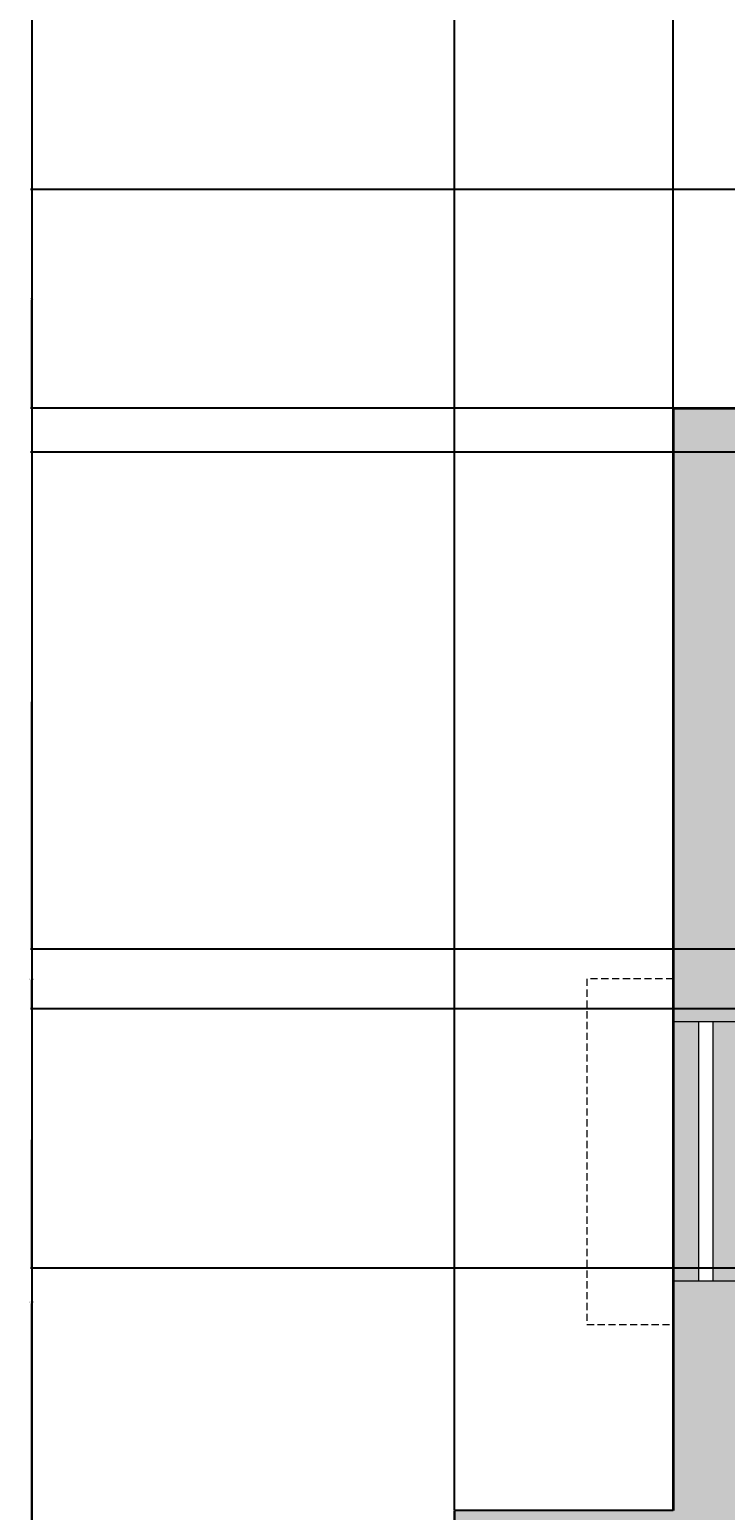
# Model space of a CAD drawing. Units: inches. Extents: x 1693 to 2974, y 2201 to 2965.
# Tile 4 of 24: x 1693 to 1790, y 2554 to 2759. Entities that reach past the tile are written whole.
import ezdxf

# ---------------------------------------------------------------- set-up
doc = ezdxf.new("R2010")
doc.units = ezdxf.units.IN
doc.header["$LTSCALE"] = 2
doc.header["$MEASUREMENT"] = 0
doc.linetypes.add('HIDDEN', pattern=[0.375, 0.25, -0.125])
for name, color, linetype, lineweight in [('A-ANNO-DIMS', 2, 'Continuous', 18), ('A-FLOR-SHFT', 7, 'Continuous', 25), ('A-GLAZ', 4, 'Continuous', 18), ('A-GLAZ-OVHD', 8, 'HIDDEN', 13), ('A-WALL', 7, 'Continuous', 35)]:
    doc.layers.add(name, color=color, linetype=linetype, lineweight=lineweight)
doc.layers.add('A-GLAZ-PATT', color=141, linetype='Continuous', lineweight=13, true_color=0xadddf7)
doc.layers.add('A-WALL-PATT', color=251, linetype='Continuous', lineweight=13, true_color=0x636466)
doc.styles.get("Standard").update_dxf_attribs({"font": 'arial.ttf'})
doc.dimstyles.get("Standard").update_dxf_attribs({"dimtxt": 0.18, "dimasz": 0.18, "dimexe": 0.18, "dimexo": 0.0625, "dimgap": 0.09, "dimtad": 0, "dimtih": 1, "dimtoh": 1, "dimdec": 1, "dimzin": 0, "dimdsep": 46, "dimlunit": 3, "dimtxsty": 'Standard', "dimcen": 0.09, "dimadec": 0, "dimazin": 0, "dimtfac": 1, "dimtdec": 1, "dimtofl": 0, "dimtmove": 0, "dimatfit": 3, "dimfxl": 1, "dimtolj": 1, "dimtzin": 0, "dimarcsym": 0})

# ---------------------------------------------------------------- blocks, each defined once
blk = doc.blocks.new('WINDOW-HOOD-48IN')
at = {"ltscale": 2}
for p, q in [((12, 48), (0, 48)), ((0, 48), (0, 6)), ((12, 42), (12, 48)), ((0, 6), (0, 0)), ((0, 0), (12, 0))]:
    blk.add_line(p, q, dxfattribs=at)
blk = doc.blocks.new('*D81')
at = {"layer": 'A-ANNO-DIMS', "color": 0, "lineweight": -2, "ltscale": 2, "transparency": 16777216}
for p, q in [((1752.34, 2553.91), (1752.34, 2964.96)), ((1752.52, 2964.78), (2332.94, 2964.78)), ((2914.06, 2964.78), (2333.64, 2964.78)), ((2914.24, 2754.97), (2914.24, 2964.96))]:
    blk.add_line(p, q, dxfattribs=at)
at = {"layer": 'A-ANNO-DIMS', "color": 0, "ltscale": 2, "transparency": 16777216}
for points in [[(1752.52, 2964.81), (1752.52, 2964.75), (1752.34, 2964.78)], [(2914.06, 2964.81), (2914.06, 2964.75), (2914.24, 2964.78)]]:
    blk.add_solid(points, dxfattribs=at)
at = {"layer": 'Defpoints', "color": 0, "ltscale": 2, "transparency": 16777216}
for p in [(2914.24, 2964.78), (2914.24, 2754.9), (1752.34, 2553.84)]:
    blk.add_point(p, dxfattribs=at)
at = {"layer": 'A-ANNO-DIMS', "color": 0, "ltscale": 2, "transparency": 16777216, "insert": (2333.29, 2964.78), "char_height": 0.18, "attachment_point": 5}
blk.add_mtext('\\A1;1162', dxfattribs=at)
blk = doc.blocks.new('*D82')
at = {"layer": 'A-ANNO-DIMS', "color": 0, "lineweight": -2, "ltscale": 2, "transparency": 16777216}
for p, q in [((2615.67, 2906.08), (1693.46, 2906.08)), ((1693.64, 2905.9), (1693.64, 2582.94)), ((1693.64, 2259.62), (1693.64, 2582.58)), ((2096.17, 2259.44), (1693.46, 2259.44))]:
    blk.add_line(p, q, dxfattribs=at)
at = {"layer": 'A-ANNO-DIMS', "color": 0, "ltscale": 2, "transparency": 16777216}
for points in [[(1693.61, 2905.9), (1693.67, 2905.9), (1693.64, 2906.08)], [(1693.61, 2259.62), (1693.67, 2259.62), (1693.64, 2259.44)]]:
    blk.add_solid(points, dxfattribs=at)
at = {"layer": 'Defpoints', "color": 0, "ltscale": 2, "transparency": 16777216}
for p in [(1693.64, 2906.08), (2615.74, 2906.08), (2096.24, 2259.44)]:
    blk.add_point(p, dxfattribs=at)
at = {"layer": 'A-ANNO-DIMS', "color": 0, "ltscale": 2, "transparency": 16777216, "insert": (1693.64, 2582.76), "char_height": 0.18, "attachment_point": 5}
blk.add_mtext('\\A1;646.6', dxfattribs=at)
blk = doc.blocks.new('*D86')
at = {"layer": 'A-ANNO-DIMS', "color": 0, "lineweight": -2, "ltscale": 2, "transparency": 16777216}
for p, q in [((1782.67, 2706.84), (1693.46, 2706.84)), ((1693.64, 2706.66), (1693.64, 2498.53)), ((1693.64, 2290.02), (1693.64, 2498.16)), ((1782.67, 2289.84), (1693.46, 2289.84))]:
    blk.add_line(p, q, dxfattribs=at)
at = {"layer": 'A-ANNO-DIMS', "color": 0, "ltscale": 2, "transparency": 16777216}
for points in [[(1693.61, 2706.66), (1693.67, 2706.66), (1693.64, 2706.84)], [(1693.61, 2290.02), (1693.67, 2290.02), (1693.64, 2289.84)]]:
    blk.add_solid(points, dxfattribs=at)
at = {"layer": 'Defpoints', "color": 0, "ltscale": 2, "transparency": 16777216}
for p in [(1693.64, 2706.84), (1782.74, 2706.84), (1782.74, 2289.84)]:
    blk.add_point(p, dxfattribs=at)
at = {"layer": 'A-ANNO-DIMS', "color": 0, "ltscale": 2, "transparency": 16777216, "insert": (1693.64, 2498.34), "char_height": 0.18, "attachment_point": 5}
blk.add_mtext('\\A1;417', dxfattribs=at)
blk = doc.blocks.new('*D88')
at = {"layer": 'A-ANNO-DIMS', "color": 0, "lineweight": -2, "ltscale": 2, "transparency": 16777216}
for p, q in [((2479.17, 2700.75), (1693.46, 2700.75)), ((1693.64, 2700.57), (1693.64, 2666.44)), ((1693.64, 2631.93), (1693.64, 2666.07)), ((2479.17, 2631.75), (1693.46, 2631.75))]:
    blk.add_line(p, q, dxfattribs=at)
at = {"layer": 'A-ANNO-DIMS', "color": 0, "ltscale": 2, "transparency": 16777216}
for points in [[(1693.61, 2700.57), (1693.67, 2700.57), (1693.64, 2700.75)], [(1693.61, 2631.93), (1693.67, 2631.93), (1693.64, 2631.75)]]:
    blk.add_solid(points, dxfattribs=at)
at = {"layer": 'Defpoints', "color": 0, "ltscale": 2, "transparency": 16777216}
for p in [(1693.64, 2700.75), (2479.24, 2700.75), (2479.24, 2631.75)]:
    blk.add_point(p, dxfattribs=at)
at = {"layer": 'A-ANNO-DIMS', "color": 0, "ltscale": 2, "transparency": 16777216, "insert": (1693.64, 2666.25), "char_height": 0.18, "attachment_point": 5}
blk.add_mtext('\\A1;69', dxfattribs=at)
blk = doc.blocks.new('*D98')
at = {"layer": 'A-ANNO-DIMS', "color": 0, "lineweight": -2, "ltscale": 2, "transparency": 16777216}
for p, q in [((2479.17, 2623.46), (1693.46, 2623.46)), ((1693.64, 2623.28), (1693.64, 2605.64)), ((1693.64, 2587.64), (1693.64, 2605.28)), ((2479.17, 2587.46), (1693.46, 2587.46))]:
    blk.add_line(p, q, dxfattribs=at)
at = {"layer": 'A-ANNO-DIMS', "color": 0, "ltscale": 2, "transparency": 16777216}
for points in [[(1693.61, 2623.28), (1693.67, 2623.28), (1693.64, 2623.46)], [(1693.61, 2587.64), (1693.67, 2587.64), (1693.64, 2587.46)]]:
    blk.add_solid(points, dxfattribs=at)
at = {"layer": 'Defpoints', "color": 0, "ltscale": 2, "transparency": 16777216}
for p in [(1693.64, 2623.46), (2479.24, 2623.46), (2479.24, 2587.46)]:
    blk.add_point(p, dxfattribs=at)
at = {"layer": 'A-ANNO-DIMS', "color": 0, "ltscale": 2, "transparency": 16777216, "insert": (1693.64, 2605.46), "char_height": 0.18, "attachment_point": 5}
blk.add_mtext('\\A1;36', dxfattribs=at)
blk = doc.blocks.new('*D99')
at = {"layer": 'A-ANNO-DIMS', "color": 0, "lineweight": -2, "ltscale": 2, "transparency": 16777216}
for p, q in [((2479.17, 2631.75), (1693.46, 2631.75)), ((1693.64, 2631.57), (1693.64, 2627.79)), ((1693.64, 2623.64), (1693.64, 2627.43)), ((2479.17, 2623.46), (1693.46, 2623.46))]:
    blk.add_line(p, q, dxfattribs=at)
at = {"layer": 'A-ANNO-DIMS', "color": 0, "ltscale": 2, "transparency": 16777216}
for points in [[(1693.61, 2631.57), (1693.67, 2631.57), (1693.64, 2631.75)], [(1693.61, 2623.64), (1693.67, 2623.64), (1693.64, 2623.46)]]:
    blk.add_solid(points, dxfattribs=at)
at = {"layer": 'Defpoints', "color": 0, "ltscale": 2, "transparency": 16777216}
for p in [(1693.64, 2631.75), (2479.24, 2631.75), (2479.24, 2623.46)]:
    blk.add_point(p, dxfattribs=at)
at = {"layer": 'A-ANNO-DIMS', "color": 0, "ltscale": 2, "transparency": 16777216, "insert": (1693.64, 2627.61), "char_height": 0.18, "attachment_point": 5}
blk.add_mtext('\\A1;8.295', dxfattribs=at)
blk = doc.blocks.new('*D102')
at = {"layer": 'A-ANNO-DIMS', "color": 0, "lineweight": -2, "ltscale": 2, "transparency": 16777216}
for p, q in [((1782.74, 2706.91), (1782.74, 2964.96)), ((1782.92, 2964.78), (1852.97, 2964.78)), ((1923.56, 2964.78), (1853.5, 2964.78)), ((1923.74, 2706.91), (1923.74, 2964.96))]:
    blk.add_line(p, q, dxfattribs=at)
at = {"layer": 'A-ANNO-DIMS', "color": 0, "ltscale": 2, "transparency": 16777216}
for points in [[(1782.92, 2964.81), (1782.92, 2964.75), (1782.74, 2964.78)], [(1923.56, 2964.81), (1923.56, 2964.75), (1923.74, 2964.78)]]:
    blk.add_solid(points, dxfattribs=at)
at = {"layer": 'Defpoints', "color": 0, "ltscale": 2, "transparency": 16777216}
for p in [(1923.74, 2964.78), (1782.74, 2706.84), (1923.74, 2706.84)]:
    blk.add_point(p, dxfattribs=at)
at = {"layer": 'A-ANNO-DIMS', "color": 0, "ltscale": 2, "transparency": 16777216, "insert": (1853.24, 2964.78), "char_height": 0.18, "attachment_point": 5}
blk.add_mtext('\\A1;141', dxfattribs=at)
blk = doc.blocks.new('*D105')
at = {"layer": 'A-ANNO-DIMS', "color": 0, "lineweight": -2, "ltscale": 2, "transparency": 16777216}
for p, q in [((1923.67, 2737.22), (1693.46, 2737.22)), ((1693.64, 2737.04), (1693.64, 2722.21)), ((1693.64, 2707.02), (1693.64, 2721.85)), ((1923.67, 2706.84), (1693.46, 2706.84))]:
    blk.add_line(p, q, dxfattribs=at)
at = {"layer": 'A-ANNO-DIMS', "color": 0, "ltscale": 2, "transparency": 16777216}
for points in [[(1693.61, 2737.04), (1693.67, 2737.04), (1693.64, 2737.22)], [(1693.61, 2707.02), (1693.67, 2707.02), (1693.64, 2706.84)]]:
    blk.add_solid(points, dxfattribs=at)
at = {"layer": 'Defpoints', "color": 0, "ltscale": 2, "transparency": 16777216}
for p in [(1693.64, 2737.22), (1923.74, 2737.22), (1923.74, 2706.84)]:
    blk.add_point(p, dxfattribs=at)
at = {"layer": 'A-ANNO-DIMS', "color": 0, "ltscale": 2, "transparency": 16777216, "insert": (1693.64, 2722.03), "char_height": 0.18, "attachment_point": 5}
blk.add_mtext('\\A1;30.37', dxfattribs=at)

msp = doc.modelspace()

# ---------------------------------------------------------------- hatches: boundary and pattern name
at = {"layer": 'A-GLAZ-PATT', "ltscale": 2}
h = msp.add_hatch(color=256, dxfattribs=at)
h.dxf.hatch_style = 1
h.paths.add_polyline_path([(2656.9702, 2338.2547), (2632.9702, 2338.2547), (2632.9702, 2339.2547), (2608.9702, 2339.2547), (2608.9702, 2334.7547), (2656.9702, 2334.7547)])
h.paths.add_polyline_path([(2656.9702, 2343.7547), (2608.9702, 2343.7547), (2608.9702, 2340.2547), (2632.9702, 2340.2547), (2632.9702, 2339.2547), (2656.9702, 2339.2547)])
h.paths.add_polyline_path([(2775.7544, 2338.2547), (2751.7544, 2338.2547), (2751.7544, 2334.7547), (2775.7544, 2334.7547)])
h.paths.add_polyline_path([(2775.7544, 2343.7547), (2751.7544, 2343.7547), (2751.7544, 2340.2547), (2775.7544, 2340.2547)])
h.paths.add_polyline_path([(2897.7363, 2568.7999), (2893.2363, 2568.7999), (2893.2363, 2520.7999), (2896.7363, 2520.7999), (2896.7363, 2544.7999), (2897.7363, 2544.7999)])
h.paths.add_polyline_path([(2902.2363, 2568.7999), (2898.7363, 2568.7999), (2898.7363, 2544.7999), (2897.7363, 2544.7999), (2897.7363, 2520.7999), (2902.2363, 2520.7999)])
h.paths.add_polyline_path([(2902.2363, 2637.7547), (2898.7363, 2637.7547), (2898.7363, 2613.7547), (2902.2363, 2613.7547)])
h.paths.add_polyline_path([(2896.7363, 2637.7547), (2893.2363, 2637.7547), (2893.2363, 2613.7547), (2896.7363, 2613.7547)])
h.paths.add_polyline_path([(2902.2363, 2748.903), (2899.0477, 2748.903), (2899.0477, 2724.903), (2898.0477, 2724.903), (2898.0477, 2700.903), (2902.2363, 2700.903)])
h.paths.add_polyline_path([(2898.0477, 2748.903), (2893.2363, 2748.903), (2893.2363, 2700.903), (2897.0477, 2700.903), (2897.0477, 2724.903), (2898.0477, 2724.903)])
h.paths.add_polyline_path([(2851.2363, 2846.2547), (2803.2363, 2846.2547), (2803.2363, 2842.7547), (2827.2363, 2842.7547), (2827.2363, 2841.7547), (2851.2363, 2841.7547)])
h.paths.add_polyline_path([(2851.2363, 2840.7547), (2827.2363, 2840.7547), (2827.2363, 2841.7547), (2803.2363, 2841.7547), (2803.2363, 2837.2547), (2851.2363, 2837.2547)])
h.paths.add_polyline_path([(2578.2363, 2846.2547), (2530.2363, 2846.2547), (2530.2363, 2842.7547), (2554.2363, 2842.7547), (2554.2363, 2841.7547), (2578.2363, 2841.7547)])
h.paths.add_polyline_path([(2578.2363, 2840.7547), (2554.2363, 2840.7547), (2554.2363, 2841.7547), (2530.2363, 2841.7547), (2530.2363, 2837.2547), (2578.2363, 2837.2547)])
h.paths.add_polyline_path([(2732.7363, 2812.7547), (2705.1363, 2812.7547), (2705.1363, 2811.7547), (2676.3363, 2811.7547), (2676.3363, 2812.7547), (2648.7363, 2812.7547), (2648.7363, 2808.2547), (2732.7363, 2808.2547)])
h.paths.add_polyline_path([(2732.7363, 2817.2547), (2648.7363, 2817.2547), (2648.7363, 2813.7547), (2676.3363, 2813.7547), (2676.3363, 2812.7547), (2705.1363, 2812.7547), (2705.1363, 2813.7547), (2732.7363, 2813.7547)])
h.paths.add_polyline_path([(2488.2363, 2695.8203), (2484.7878, 2695.8203), (2484.7878, 2671.8203), (2488.2363, 2671.8203)])
h.paths.add_polyline_path([(2482.7878, 2695.8203), (2479.2363, 2695.8203), (2479.2363, 2671.8203), (2482.7878, 2671.8203)])
h.paths.add_polyline_path([(2488.2363, 2572.4371), (2484.7363, 2572.4371), (2484.7363, 2541.4371), (2483.7363, 2541.4371), (2483.7363, 2512.4371), (2488.2363, 2512.4371)])
h.paths.add_polyline_path([(2482.7363, 2541.4371), (2483.7363, 2541.4371), (2483.7363, 2572.4371), (2479.2363, 2572.4371), (2479.2363, 2512.4371), (2482.7363, 2512.4371)])
h.paths.add_polyline_path([(2248.9863, 2706.8449), (2190.9863, 2706.8449), (2190.9863, 2703.3449), (2219.9863, 2703.3449), (2219.9863, 2702.3449), (2248.9863, 2702.3449)])
h.paths.add_polyline_path([(2248.9863, 2701.3449), (2219.9863, 2701.3449), (2219.9863, 2702.3449), (2190.9863, 2702.3449), (2190.9863, 2697.8449), (2248.9863, 2697.8449)])
h.paths.add_polyline_path([(2151.9207, 2293.3449), (2127.9207, 2293.3449), (2127.9207, 2289.8449), (2151.9207, 2289.8449)])
h.paths.add_polyline_path([(2151.9207, 2298.8449), (2127.9207, 2298.8449), (2127.9207, 2295.3449), (2151.9207, 2295.3449)])
h.paths.add_polyline_path([(2084.023, 2293.3449), (2066.023, 2293.3449), (2066.023, 2294.3449), (2048.023, 2294.3449), (2048.023, 2289.8449), (2084.023, 2289.8449)])
h.paths.add_polyline_path([(2084.023, 2298.8449), (2048.023, 2298.8449), (2048.023, 2295.3449), (2066.023, 2295.3449), (2066.023, 2294.3449), (2084.023, 2294.3449)])
h.paths.add_polyline_path([(1966.0781, 2293.3449), (1948.0781, 2293.3449), (1948.0781, 2294.3449), (1930.0781, 2294.3449), (1930.0781, 2289.8449), (1966.0781, 2289.8449)])
h.paths.add_polyline_path([(1966.0781, 2298.8449), (1930.0781, 2298.8449), (1930.0781, 2295.3449), (1948.0781, 2295.3449), (1948.0781, 2294.3449), (1966.0781, 2294.3449)])
h.paths.add_polyline_path([(1787.2363, 2403.1922), (1782.7363, 2403.1922), (1782.7363, 2355.1922), (1786.2363, 2355.1922), (1786.2363, 2379.1922), (1787.2363, 2379.1922)])
h.paths.add_polyline_path([(1791.7363, 2403.1922), (1788.2363, 2403.1922), (1788.2363, 2379.1922), (1787.2363, 2379.1922), (1787.2363, 2355.1922), (1791.7363, 2355.1922)])
h.paths.add_polyline_path([(1786.2363, 2477.5455), (1782.7363, 2477.5455), (1782.7363, 2453.5455), (1786.2363, 2453.5455)])
h.paths.add_polyline_path([(1791.7363, 2477.5455), (1788.2363, 2477.5455), (1788.2363, 2453.5455), (1791.7363, 2453.5455)])
h.paths.add_polyline_path([(1786.2363, 2621.6433), (1782.7363, 2621.6433), (1782.7363, 2585.6433), (1786.2363, 2585.6433)])
h.paths.add_polyline_path([(1791.7363, 2621.6433), (1788.2363, 2621.6433), (1788.2363, 2585.6433), (1791.7363, 2585.6433)])
h.paths.add_polyline_path([(1908.1286, 2706.8449), (1860.1286, 2706.8449), (1860.1286, 2703.3449), (1884.1286, 2703.3449), (1884.1286, 2702.3449), (1908.1286, 2702.3449)])
h.paths.add_polyline_path([(1908.1286, 2701.3449), (1884.1286, 2701.3449), (1884.1286, 2702.3449), (1860.1286, 2702.3449), (1860.1286, 2697.8449), (1908.1286, 2697.8449)])
h.paths.add_polyline_path([(1973.9863, 2706.8449), (1949.9863, 2706.8449), (1949.9863, 2703.3449), (1973.9863, 2703.3449)])
h.paths.add_polyline_path([(1973.9863, 2701.3449), (1949.9863, 2701.3449), (1949.9863, 2697.8449), (1973.9863, 2697.8449)])
h.paths.add_polyline_path([(2112.7363, 2690.3449), (2028.7363, 2690.3449), (2028.7363, 2686.8449), (2056.3363, 2686.8449), (2056.3363, 2685.8449), (2085.1363, 2685.8449), (2085.1363, 2686.8449), (2112.7363, 2686.8449)])
h.paths.add_polyline_path([(2112.7363, 2685.8449), (2085.1363, 2685.8449), (2085.1363, 2684.8449), (2056.3363, 2684.8449), (2056.3363, 2685.8449), (2028.7363, 2685.8449), (2028.7363, 2681.3449), (2112.7363, 2681.3449)])
h.paths.add_polyline_path([(2422.7363, 2640.7547), (2350.7363, 2640.7547), (2350.7363, 2637.2547), (2386.7363, 2637.2547), (2386.7363, 2636.2547), (2422.7363, 2636.2547)])
h.paths.add_polyline_path([(2422.7363, 2635.2547), (2386.7363, 2635.2547), (2386.7363, 2636.2547), (2350.7363, 2636.2547), (2350.7363, 2631.7547), (2422.7363, 2631.7547)])
at = {"layer": 'A-WALL-PATT', "ltscale": 2}
h = msp.add_hatch(color=256, dxfattribs=at)
h.dxf.hatch_style = 1
h.paths.add_polyline_path([(1928.2363, 2733.2161), (1930.9384, 2733.2161), (1930.9384, 2737.2161), (1923.7363, 2737.2161), (1923.7363, 2706.8449), (1908.1286, 2706.8449), (1908.1286, 2697.8449), (1923.7363, 2697.8449), (1923.7363, 2692.8449), (1928.2363, 2692.8449), (1928.2363, 2697.8449), (1949.9863, 2697.8449), (1949.9863, 2706.8449), (1928.2363, 2706.8449)])
h.paths.add_polyline_path([(2004.7363, 2737.2161), (1995.7363, 2737.2161), (1995.7363, 2706.8449), (1985.6374, 2706.8449), (1973.9863, 2706.8449), (1973.9863, 2697.8449), (2000.2363, 2697.8449), (2000.2363, 2686.5348), (2000.3613, 2686.5348), (2000.3613, 2667.0432), (2000.2363, 2601.8449), (1928.2363, 2601.8449), (1928.2363, 2662.8449), (1923.7363, 2662.8449), (1923.7363, 2595.3449), (1928.2363, 2595.3449), (1928.2363, 2597.3449), (2004.7363, 2597.3449), (2004.7363, 2681.3449), (2012.7814, 2681.3449), (2028.7363, 2681.3449), (2028.7363, 2690.3449), (2004.7363, 2690.3449)])
h.paths.add_polyline_path([(2190.9863, 2706.8449), (2184.9863, 2706.8449), (2145.7363, 2706.8449), (2145.7363, 2765.3449), (2145.7363, 2774.5394), (2136.7363, 2774.5394), (2136.7363, 2756.3449), (2136.7363, 2690.3449), (2112.7363, 2690.3449), (2112.7363, 2681.3449), (2136.7363, 2681.3449), (2136.7363, 2597.3449), (2141.2363, 2597.3449), (2141.2363, 2697.8449), (2190.9863, 2697.8449)])
h.paths.add_polyline_path([(1860.1286, 2706.8449), (1782.7363, 2706.8449), (1782.7363, 2621.6433), (1791.7363, 2621.6433), (1791.7363, 2697.8449), (1860.1286, 2697.8449)])
h.paths.add_polyline_path([(1791.7363, 2585.6433), (1782.7363, 2585.6433), (1782.7363, 2562.8449), (1782.7363, 2553.8449), (1752.3363, 2553.8449), (1752.3363, 2544.2586), (1756.3363, 2544.2586), (1756.3363, 2549.3449), (1782.7363, 2549.3449), (1782.7363, 2489.2404), (1782.7363, 2477.5455), (1791.7363, 2477.5455), (1791.7363, 2493.5991), (1791.6113, 2493.5991), (1791.6113, 2513.0907), (1791.6824, 2533.7198, -0.94742783), (1791.7363, 2534.7168), (1791.7363, 2549.3449), (1863.7363, 2549.3449), (1863.7363, 2513.3449), (1866.7363, 2513.3449), (1866.7363, 2549.3449), (1924.7363, 2549.3449), (1924.7363, 2447.3449), (1924.7363, 2442.8449), (1933.7363, 2442.8449), (1933.7363, 2447.3449), (1928.2363, 2447.3449), (1928.2363, 2559.3449), (1923.7363, 2559.3449), (1923.7363, 2553.8449), (1791.7363, 2553.8449), (1791.7363, 2562.8449)])
h.paths.add_polyline_path([(1791.7363, 2442.8449), (1866.7363, 2442.8449), (1866.7363, 2447.3449), (1866.7363, 2483.3449), (1863.7363, 2483.3449), (1863.7363, 2447.3449), (1791.7363, 2447.3449), (1791.7363, 2453.5455), (1782.7363, 2453.5455), (1782.7363, 2447.3449), (1756.3363, 2447.3449), (1756.3363, 2455.7126), (1752.3363, 2455.7126), (1752.3363, 2442.8449), (1782.7363, 2442.8449), (1782.7363, 2403.1922), (1791.7363, 2403.1922)])
h.paths.add_polyline_path([(1930.0781, 2298.8449), (1791.7363, 2298.8449), (1791.7363, 2355.1922), (1782.7363, 2355.1922), (1782.7363, 2289.8449), (1930.0781, 2289.8449)])
h.paths.add_polyline_path([(2624.7363, 2883.2547), (2624.7363, 2902.6165), (2624.7363, 2906.0761), (2615.7363, 2906.0761), (2615.7363, 2892.2547), (2615.7363, 2846.2547), (2578.2363, 2846.2547), (2578.2363, 2837.2547), (2620.2363, 2837.2547), (2620.2363, 2743.2547), (2624.7363, 2743.2547), (2624.7363, 2808.2547), (2648.7363, 2808.2547), (2648.7363, 2817.2547), (2624.7363, 2817.2547)])
h.paths.add_polyline_path([(2530.2363, 2846.2547), (2479.2363, 2846.2547), (2479.2363, 2695.8203), (2488.2363, 2695.8203), (2488.2363, 2700.7547), (2567.2363, 2700.7547), (2567.2363, 2705.2547), (2488.2363, 2705.2547), (2488.2363, 2837.2547), (2530.2363, 2837.2547)])
h.paths.add_polyline_path([(2488.2363, 2487.7547), (2630.2363, 2487.7547, -0.00990191), (2630.2363, 2489.0322), (2630.2363, 2492.2547), (2488.2363, 2492.2547), (2488.2363, 2512.4371), (2479.2363, 2512.4371), (2479.2363, 2334.7547), (2608.9702, 2334.7547), (2608.9702, 2343.7547), (2488.2363, 2343.7547)])
h.paths.add_polyline_path([(2751.7544, 2343.7547), (2672.7363, 2343.7547), (2672.7363, 2409.7547), (2674.7363, 2409.7547), (2674.7363, 2413.7547), (2672.7363, 2413.7547), (2672.7363, 2487.7547), (2732.7363, 2487.7547), (2732.7363, 2413.7547), (2704.7363, 2413.7547), (2704.7363, 2409.7547), (2784.7363, 2409.7547), (2784.7363, 2343.7547), (2775.7544, 2343.7547), (2775.7544, 2334.7547), (2902.2363, 2334.7547), (2902.2363, 2520.7999), (2893.2363, 2520.7999), (2893.2363, 2413.7547), (2856.0145, 2413.7547), (2856.0145, 2409.7547), (2893.2363, 2409.7547), (2893.2363, 2343.7547), (2789.2363, 2343.7547), (2789.2363, 2409.7547), (2819.2363, 2409.7547), (2826.0145, 2409.7547), (2826.0145, 2413.7547), (2789.2363, 2413.7547), (2789.2363, 2492.2547), (2784.7363, 2492.2547), (2784.7363, 2413.7547), (2736.7363, 2413.7547), (2736.7363, 2492.2547), (2672.7363, 2492.2547), (2666.2363, 2492.2547), (2666.2363, 2487.7547), (2668.2363, 2487.7547), (2668.2363, 2343.7547), (2656.9702, 2343.7547), (2656.9702, 2334.7547), (2662.9702, 2334.7547), (2751.7544, 2334.7547)])
h.paths.add_polyline_path([(2902.2363, 2613.7547), (2893.2363, 2613.7547), (2893.2363, 2589.7547), (2785.2363, 2589.7547), (2785.2363, 2661.7547), (2790.2363, 2661.7547), (2790.2363, 2665.2547), (2761.2363, 2665.2547), (2761.2363, 2667.2547), (2756.7363, 2667.2547), (2756.7363, 2661.7547), (2781.2363, 2661.7547), (2781.2363, 2585.7547), (2893.2363, 2585.7547), (2893.2363, 2568.7999), (2902.2363, 2568.7999)])
h.paths.add_polyline_path([(2488.2363, 2671.8203), (2479.2363, 2671.8203), (2479.2363, 2645.2547), (2479.2363, 2623.4598), (2488.2363, 2623.4598), (2488.2363, 2636.2547), (2624.7363, 2636.2547), (2624.7363, 2640.7547), (2603.7363, 2640.7547), (2603.7363, 2700.7547), (2624.7363, 2700.7547), (2624.7363, 2707.2547), (2620.2363, 2707.2547), (2620.2363, 2705.2547), (2597.2363, 2705.2547), (2597.2363, 2700.7547), (2599.2363, 2700.7547), (2599.2363, 2640.7547), (2488.2363, 2640.7547)])
h.paths.add_polyline_path([(2761.2363, 2837.2547), (2803.2363, 2837.2547), (2803.2363, 2846.2547), (2797.2363, 2846.2547), (2765.7363, 2846.2547), (2756.7363, 2846.2547), (2756.7363, 2817.2547), (2732.7363, 2817.2547), (2732.7363, 2808.2547), (2756.7363, 2808.2547), (2756.7363, 2703.2547), (2761.2363, 2703.2547)])
h.paths.add_polyline_path([(2739.7489, 2433.1234), (2786.9181, 2433.1234), (2786.9181, 2455.5122), (2739.7489, 2455.5122)], flags=25)

# ---------------------------------------------------------------- linework, layer by layer
at = {"layer": 'A-FLOR-SHFT', "ltscale": 2}
for p, q in [((1782.7363, 2553.8449), (1752.3363, 2553.8449)), ((1752.3363, 2553.8449), (1752.3363, 2544.2586)), ((1752.3363, 2544.2586), (1752.3363, 2553.8449))]:
    msp.add_line(p, q, dxfattribs=at)
at = {"layer": 'A-GLAZ', "ltscale": 2}
for p, q in [((1791.7363, 2621.6433), (1782.7363, 2621.6433)), ((1786.2363, 2621.6433), (1786.2363, 2585.6433)), ((1788.2363, 2621.6433), (1788.2363, 2585.6433)), ((1791.7363, 2585.6433), (1782.7363, 2585.6433))]:
    msp.add_line(p, q, dxfattribs=at)
at = {"layer": 'A-WALL'}
for p, q in [((1782.7363, 2706.8449), (1923.7363, 2706.8449)), ((1782.7363, 2706.8449), (1782.7363, 2562.8449)), ((1782.7363, 2571.1208), (1782.7363, 2553.8449))]:
    msp.add_line(p, q, dxfattribs=at)

# ---------------------------------------------------------------- block references
at = {"layer": 'A-GLAZ-OVHD'}
msp.add_blockref('WINDOW-HOOD-48IN', (1770.736, 2579.643), dxfattribs=at)

# ---------------------------------------------------------------- dimensions: what is measured, and where the dimension line sits
at = {"layer": 'A-ANNO-DIMS', "ltscale": 2}
for base, p1, p2, picture, middle in [((2914.2363, 2964.7761), (1752.3363, 2553.8449), (2914.2363, 2754.903), '*D81', (2333.2863, 2964.7761)), ((1923.7363, 2964.7761), (1782.7363, 2706.8449), (1923.7363, 2706.8449), '*D102', (1853.2363, 2964.7761))]:
    dim = msp.add_linear_dim(base=base, p1=p1, p2=p2, dimstyle='Standard', override={"dimdec": 0, "dimlfac": 1, "dimrnd": 0, "dimzin": 0, "dimdsep": 46, "dimlunit": 2}, dxfattribs=at)
    dim.commit()
    dim.dimension.update_dxf_attribs({"geometry": picture, "text_midpoint": middle})
for base, p1, p2, override, picture, middle in [((1693.6363, 2906.0761), (2096.2363, 2259.4449), (2615.7363, 2906.0761), {"dimdec": 1, "dimlfac": 1, "dimrnd": 0, "dimzin": 0, "dimdsep": 46, "dimlunit": 2}, '*D82', (1693.6363, 2582.7605)), ((1693.6363, 2737.2161), (1923.7363, 2706.8449), (1923.7363, 2737.2161), {"dimdec": 2, "dimlfac": 1, "dimrnd": 0, "dimzin": 0, "dimdsep": 46, "dimlunit": 2}, '*D105', (1693.6363, 2722.0305)), ((1693.6363, 2706.8449), (1782.7363, 2289.8449), (1782.7363, 2706.8449), {"dimdec": 0, "dimlfac": 1, "dimrnd": 0, "dimzin": 0, "dimdsep": 46, "dimlunit": 2}, '*D86', (1693.6363, 2498.3449)), ((1693.6363, 2700.7547), (2479.2363, 2631.7547), (2479.2363, 2700.7547), {"dimdec": 0, "dimlfac": 1, "dimrnd": 0, "dimzin": 0, "dimdsep": 46, "dimlunit": 2}, '*D88', (1693.6363, 2666.2547)), ((1693.6363, 2631.7547), (2479.2363, 2623.4598), (2479.2363, 2631.7547), {"dimdec": 3, "dimlfac": 1, "dimrnd": 0, "dimzin": 0, "dimdsep": 46, "dimlunit": 2}, '*D99', (1693.6363, 2627.6073)), ((1693.6363, 2623.4598), (2479.2363, 2587.4598), (2479.2363, 2623.4598), {"dimdec": 0, "dimlfac": 1, "dimrnd": 0, "dimzin": 0, "dimdsep": 46, "dimlunit": 2}, '*D98', (1693.6363, 2605.4598))]:
    dim = msp.add_linear_dim(base=base, p1=p1, p2=p2, angle=90, dimstyle='Standard', override=override, dxfattribs=at)
    dim.commit()
    dim.dimension.update_dxf_attribs({"geometry": picture, "text_midpoint": middle})

doc.saveas('drawing.dxf')
